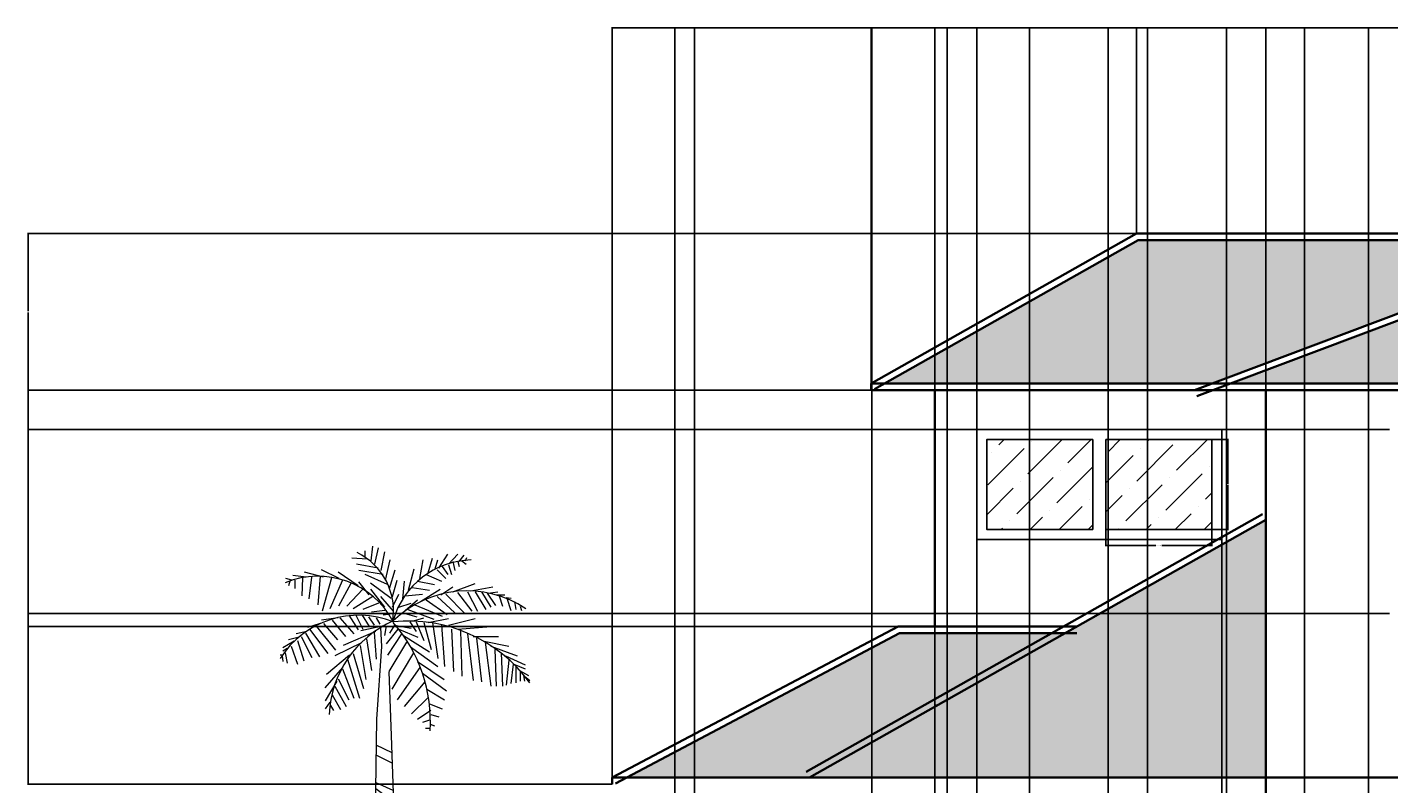
# Model space of a CAD drawing. Units: inches. Extents: x -177 to 697, y -125 to 346.
# Tile 2 of 4: x -177 to 237, y 116 to 346. Entities that reach past the tile are written whole.
import ezdxf

# ---------------------------------------------------------------- set-up
doc = ezdxf.new("R2010")
doc.units = ezdxf.units.IN
doc.header["$MEASUREMENT"] = 0
for name, color, linetype, lineweight in [('A-ANNO-DIMS', 2, 'Continuous', 18), ('A-GLAZ', 4, 'Continuous', 25), ('A-GLAZ-PATT', 252, 'Continuous', 13), ('A-ROOF', 1, 'Continuous', 35), ('A-ROOF-PATT', 252, 'Continuous', 13), ('A-WALL', 7, 'Continuous', 35), ('L-PLNT', 94, 'Continuous', 13)]:
    doc.layers.add(name, color=color, linetype=linetype, lineweight=lineweight)
doc.styles.get("Standard").update_dxf_attribs({"font": 'arial.ttf'})
doc.dimstyles.get("Standard").update_dxf_attribs({"dimtxt": 0.18, "dimasz": 0.18, "dimexe": 0.18, "dimexo": 0.0625, "dimgap": 0.09, "dimtad": 0, "dimtih": 1, "dimtoh": 1, "dimdec": 4, "dimzin": 0, "dimdsep": 46, "dimtxsty": 'Standard', "dimcen": 0.09, "dimadec": 0, "dimazin": 0, "dimtfac": 1, "dimtdec": 4, "dimtofl": 0, "dimtmove": 0, "dimatfit": 3, "dimfxl": 1, "dimtolj": 1, "dimtzin": 0, "dimarcsym": 0})

# ---------------------------------------------------------------- blocks, each defined once
blk = doc.blocks.new('*U2')
for p, q in [((-7.5, 199.68), (-7.5, 197.946)), ((-5.567, 196.707), (-4.987, 201.167)), ((-4.407, 195.716), (-3.247, 200.672)), ((-2.474, 193.733), (-1.315, 199.433)), ((-6.727, 197.202), (-11.366, 197.45)), ((-3.441, 194.477), (-10.013, 195.716)), ((-1.121, 190.759), (0.232, 196.955)), ((9.317, 191.255), (10.283, 196.955)), ((11.829, 192.99), (13.182, 197.45)), ((13.956, 194.229), (14.729, 196.955)), ((15.116, 194.477), (17.822, 198.689)), ((16.082, 194.972), (17.822, 192.494)), ((18.015, 195.716), (20.914, 198.689)), ((18.015, 195.468), (18.981, 192.494)), ((19.368, 196.459), (19.948, 193.733)), ((20.914, 196.459), (21.301, 194.972)), ((21.301, 196.459), (22.847, 198.441)), ((22.074, 196.707), (23.427, 195.716)), ((23.234, 196.707), (23.62, 197.698)), ((-29.729, 190.759), (-31.469, 191.255)), ((-25.283, 191.751), (-29.342, 192.246)), ((-28.763, 190.759), (-28.763, 188.281)), ((-26.443, 191.503), (-26.636, 186.051)), ((-20.064, 191.751), (-25.863, 193.238)), ((-23.737, 191.751), (-24.51, 185.06)), ((-21.031, 191.998), (-21.804, 183.325)), ((-15.232, 191.255), (-20.644, 193.981)), ((-17.551, 191.503), (-20.451, 181.343)), ((-14.265, 190.759), (-18.131, 182.086)), ((-9.433, 189.025), (-15.618, 193.238)), ((-1.894, 192.494), (-9.24, 193.733)), ((-0.541, 189.52), (-7.307, 192.494)), ((0.038, 188.281), (1.778, 193.981)), ((1.005, 185.803), (2.358, 190.759)), ((5.837, 187.786), (7.577, 194.229)), ((11.25, 192.494), (15.889, 190.512)), ((14.536, 193.981), (17.242, 191.255)), ((-30.309, 190.512), (-30.695, 189.025)), ((-11.753, 189.768), (-15.425, 182.83)), ((-8.08, 188.034), (-12.912, 182.83)), ((-6.147, 186.299), (-9.24, 190.264)), ((-5.76, 190.016), (0.618, 185.308)), ((-5.76, 188.034), (-1.508, 182.582)), ((4.098, 185.06), (4.678, 190.512)), ((6.997, 188.529), (12.216, 187.786)), ((8.544, 190.512), (13.763, 189.52)), ((9.51, 184.317), (15.502, 188.034)), ((15.695, 186.299), (19.368, 188.777)), ((19.368, 187.29), (26.133, 189.768)), ((20.721, 187.042), (25.167, 181.343)), ((23.814, 187.29), (26.907, 181.343)), ((24.78, 187.538), (31.546, 188.777)), ((26.133, 187.29), (29.419, 181.838)), ((28.066, 187.29), (30.966, 182.582)), ((29.806, 186.795), (32.319, 183.078)), ((29.999, 186.795), (33.092, 187.29)), ((-4.987, 185.803), (-10.979, 182.086)), ((-3.247, 183.821), (-8.08, 181.838)), ((-2.668, 185.803), (1.198, 181.343)), ((1.005, 182.582), (2.938, 186.547)), ((2.938, 182.582), (6.61, 183.821)), ((4.871, 186.051), (10.09, 186.547)), ((4.871, 181.591), (8.544, 184.812)), ((7.77, 183.325), (16.082, 179.856)), ((11.25, 184.812), (17.628, 180.352)), ((14.536, 185.803), (19.948, 180.847)), ((17.242, 186.547), (23.041, 180.599)), ((32.512, 186.299), (35.218, 186.299)), ((33.479, 186.051), (34.445, 182.83)), ((35.605, 185.556), (37.151, 185.308)), ((35.798, 185.308), (36.958, 181.591)), ((38.118, 184.317), (38.504, 181.838)), ((39.857, 182.83), (40.244, 181.591)), ((-15.618, 179.36), (-20.644, 178.617)), ((-17.358, 178.617), (-13.299, 173.661)), ((-15.038, 179.36), (-10.786, 174.404)), ((-12.332, 180.104), (-9.433, 175.643)), ((-10.206, 180.104), (-8.08, 175.891)), ((-8.273, 180.104), (-6.147, 176.635)), ((-6.34, 179.608), (-4.6, 177.13)), ((-1.315, 181.591), (-5.374, 181.095)), ((-4.021, 179.36), (-2.861, 177.378)), ((-0.348, 180.352), (-1.894, 180.104)), ((4.098, 180.847), (8.35, 179.608)), ((5.644, 181.838), (13.569, 178.865)), ((7.384, 178.369), (10.476, 179.36)), ((11.829, 177.874), (18.015, 179.113)), ((18.015, 177.13), (26.133, 179.113)), ((-25.09, 175.148), (-28.376, 174.404)), ((-25.476, 174.652), (-21.224, 167.466)), ((-21.031, 177.626), (-24.897, 176.387)), ((-24.317, 175.891), (-18.711, 168.457)), ((-22.191, 176.635), (-16.391, 169.448)), ((-20.064, 177.626), (-15.812, 172.67)), ((-4.214, 175.148), (-14.072, 170.935)), ((-1.701, 176.882), (-8.66, 175.396)), ((-4.6, 174.9), (-4.021, 166.722)), ((-2.668, 176.387), (-2.376, 170.594)), ((-0.928, 176.882), (-1.508, 173.909)), ((2.551, 175.891), (-0.928, 171.431)), ((3.711, 174.404), (-0.541, 167.961)), ((1.585, 177.13), (0.038, 174.652)), ((1.585, 177.13), (6.61, 176.139)), ((2.938, 175.891), (8.737, 173.413)), ((6.224, 178.121), (8.157, 175.148)), ((8.157, 178.121), (10.476, 172.422)), ((10.476, 177.874), (12.796, 169.696)), ((13.182, 177.874), (14.729, 166.97)), ((15.889, 177.13), (16.855, 164.492)), ((18.981, 175.891), (19.561, 163.005)), ((20.914, 175.891), (30.966, 176.635)), ((21.688, 175.396), (22.074, 161.518)), ((23.814, 174.404), (25.554, 160.279)), ((-28.956, 172.174), (-32.435, 170.192)), ((-27.409, 173.413), (-30.695, 172.67)), ((-29.922, 170.687), (-27.989, 165.235)), ((-27.989, 172.422), (-26.056, 166.227)), ((-26.829, 173.661), (-23.544, 167.218)), ((-8.466, 171.678), (-16.585, 167.713)), ((-8.853, 170.935), (-7.113, 160.527)), ((-6.92, 172.917), (-5.374, 163.253)), ((5.257, 171.926), (-0.155, 163.005)), ((4.291, 173.909), (12.216, 168.953)), ((6.417, 170.439), (14.729, 164.492)), ((25.554, 173.661), (33.285, 173.661)), ((26.52, 173.165), (28.066, 159.784)), ((28.839, 172.174), (36.378, 170.687)), ((29.226, 171.926), (30.966, 158.545)), ((30.966, 170.687), (38.891, 167.713)), ((-32.628, 167.961), (-33.208, 167.961)), ((-32.628, 167.713), (-32.435, 165.979)), ((-31.082, 169.944), (-32.435, 169.2)), ((-31.662, 168.705), (-31.082, 165.483)), ((-12.139, 167.961), (-19.098, 162.014)), ((-12.719, 166.722), (-9.046, 154.828)), ((-10.979, 168.457), (-7.887, 157.801)), ((7.384, 168.705), (0.812, 157.553)), ((8.544, 165.979), (16.662, 160.527)), ((32.126, 169.696), (32.512, 158.545)), ((34.058, 168.705), (34.445, 158.545)), ((35.412, 167.713), (41.404, 164.988)), ((36.378, 166.474), (35.605, 158.792)), ((-14.265, 164.244), (-19.678, 158.049)), ((-14.265, 163.749), (-10.786, 154.828)), ((9.317, 164.244), (2.358, 154.332)), ((10.09, 162.51), (17.435, 157.058)), ((37.731, 165.235), (36.958, 159.288)), ((37.924, 165.235), (41.404, 163.749)), ((38.504, 164.492), (38.504, 159.536)), ((39.664, 163.253), (42.37, 161.766)), ((39.857, 162.757), (39.857, 160.031)), ((40.824, 161.766), (41.21, 160.031)), ((-16.005, 160.031), (-19.484, 154.084)), ((-16.585, 158.545), (-13.106, 152.35)), ((-15.618, 160.775), (-12.332, 154.332)), ((10.863, 159.784), (4.484, 152.35)), ((11.443, 157.553), (16.855, 154.332)), ((41.21, 161.518), (42.757, 160.279)), ((-18.131, 153.589), (-19.484, 151.606)), ((-17.358, 155.819), (-14.845, 151.358)), ((11.829, 155.075), (6.804, 150.119)), ((-17.938, 152.597), (-16.972, 151.111)), ((12.603, 151.111), (8.544, 148.385)), ((12.216, 153.093), (16.082, 151.606)), ((12.603, 149.872), (15.116, 149.128)), ((12.216, 148.137), (10.09, 147.393)), ((12.409, 145.659), (11.056, 145.659)), ((12.409, 146.898), (13.763, 146.402)), ((-4.081, 140.645), (0.753, 138.261)), ((-4.081, 137.547), (0.753, 135.163)), ((-4.081, 129.205), (1.124, 126.821)), ((-4.081, 127.298), (1.31, 123.246)), ((-4.081, 121.578), (1.31, 120.863)), ((-4.453, 112.283), (1.682, 105.133)), ((-4.267, 114.428), (1.682, 108.708)), ((-4.639, 102.273), (1.868, 100.604)), ((-4.453, 99.651), (2.24, 98.459)), ((-4.453, 91.071), (2.426, 89.641)), ((-4.825, 83.921), (2.612, 81.061)), ((-4.639, 81.299), (2.797, 78.916)), ((-4.639, 78.916), (2.797, 76.771))]:
    blk.add_line(p, q)
for points in [[(-2.363, 170.553), (-3.88, 148.505), (-4.988, 69.634), (-3.325, 24.869), (0, 0)], [(-0.116, 162.848), (0.554, 143.532), (2.217, 96.635), (3.88, 44.054), (7.76, 12.079), (11.64, 0)]]:
    blk.add_lwpolyline(points)
for centre, radius, start, end in [((-18.427, 181.448), 19.715, 350.285, 64.11229), ((25.595, 171.567), 25.395, 91.40319, 163.882), ((-21.738, 166.094), 25.899, 27.67115, 112.5305), ((23.687, 155.341), 32.188, 56.19272, 134.3213), ((-9.259, 151.732), 28.386, 68.38311, 147.5322), ((14.394, 148.393), 32.752, 113.7592, 177.4133), ((5.828, 132.718), 45.639, 35.98777, 95.82273), ((-32.8, 147.923), 45.309, 356.1943, 41.37848)]:
    blk.add_arc(centre, radius, start, end)
blk = doc.blocks.new('WIN-SASH-UPPER-ELEV')
blk.add_line((0, 27.46), (0, 0))
blk.add_lwpolyline([(0, 27.46), (32.26, 27.46), (32.26, 0), (0, 0)])
blk = doc.blocks.new('*D13')
at = {"layer": 'A-ANNO-DIMS', "color": 0, "lineweight": -2, "transparency": 16777216}
for p, q in [((151.36, 193.16), (151.36, 188.2)), ((183.62, 193.16), (183.62, 188.2)), ((151.54, 188.38), (166.58, 188.38)), ((183.44, 188.38), (168.39, 188.38))]:
    blk.add_line(p, q, dxfattribs=at)
at = {"layer": 'A-ANNO-DIMS', "color": 0, "transparency": 16777216}
for points in [[(151.54, 188.41), (151.54, 188.35), (151.36, 188.38)], [(183.44, 188.41), (183.44, 188.35), (183.62, 188.38)]]:
    blk.add_solid(points, dxfattribs=at)
at = {"layer": 'Defpoints', "color": 0, "transparency": 16777216}
for p in [(151.36, 193.22), (183.62, 193.22), (183.62, 188.38)]:
    blk.add_point(p, dxfattribs=at)
at = {"layer": 'A-ANNO-DIMS', "color": 0, "transparency": 16777216, "insert": (167.49, 188.38), "char_height": 0.18, "attachment_point": 5}
blk.add_mtext('\\A1;SASH 32 TYP.', dxfattribs=at)
blk = doc.blocks.new('*D14')
at = {"layer": 'A-ANNO-DIMS', "color": 0, "lineweight": -2, "transparency": 16777216}
for p, q in [((183.68, 220.68), (188.64, 220.68)), ((188.46, 220.5), (188.46, 207.13)), ((188.46, 193.4), (188.46, 206.77)), ((183.68, 193.22), (188.64, 193.22))]:
    blk.add_line(p, q, dxfattribs=at)
at = {"layer": 'A-ANNO-DIMS', "color": 0, "transparency": 16777216}
for points in [[(188.43, 220.5), (188.49, 220.5), (188.46, 220.68)], [(188.43, 193.4), (188.49, 193.4), (188.46, 193.22)]]:
    blk.add_solid(points, dxfattribs=at)
at = {"layer": 'Defpoints', "color": 0, "transparency": 16777216}
for p in [(183.62, 220.68), (188.46, 220.68), (183.62, 193.22)]:
    blk.add_point(p, dxfattribs=at)
at = {"layer": 'A-ANNO-DIMS', "color": 0, "transparency": 16777216, "insert": (188.46, 206.95), "char_height": 0.18, "attachment_point": 5}
blk.add_mtext('\\A1;27 TYP.', dxfattribs=at)
blk = doc.blocks.new('*D21')
at = {"layer": 'A-ANNO-DIMS', "color": 0, "lineweight": -2, "transparency": 16777216}
for p, q in [((1.05, 117.74), (1.05, 346.22)), ((1.23, 346.04), (259.84, 346.04)), ((519.23, 346.04), (260.62, 346.04)), ((519.41, 117.74), (519.41, 346.22))]:
    blk.add_line(p, q, dxfattribs=at)
at = {"layer": 'A-ANNO-DIMS', "color": 0, "transparency": 16777216}
for points in [[(1.23, 346.07), (1.23, 346.01), (1.05, 346.04)], [(519.23, 346.07), (519.23, 346.01), (519.41, 346.04)]]:
    blk.add_solid(points, dxfattribs=at)
at = {"layer": 'Defpoints', "color": 0, "transparency": 16777216}
for p in [(519.41, 346.04), (1.05, 117.68), (519.41, 117.68)]:
    blk.add_point(p, dxfattribs=at)
at = {"layer": 'A-ANNO-DIMS', "color": 0, "transparency": 16777216, "insert": (260.23, 346.04), "char_height": 0.18, "attachment_point": 5}
blk.add_mtext('\\A1;518.4', dxfattribs=at)
blk = doc.blocks.new('*D22')
at = {"layer": 'A-ANNO-DIMS', "color": 0, "lineweight": -2, "transparency": 16777216}
for p, q in [((79.79, 235.68), (-176.98, 235.68)), ((-176.8, 235.5), (-176.8, 175.86)), ((-176.8, 115.86), (-176.8, 175.5)), ((0.99, 115.68), (-176.98, 115.68))]:
    blk.add_line(p, q, dxfattribs=at)
at = {"layer": 'A-ANNO-DIMS', "color": 0, "transparency": 16777216}
for points in [[(-176.83, 235.5), (-176.77, 235.5), (-176.8, 235.68)], [(-176.83, 115.86), (-176.77, 115.86), (-176.8, 115.68)]]:
    blk.add_solid(points, dxfattribs=at)
at = {"layer": 'Defpoints', "color": 0, "transparency": 16777216}
for p in [(79.85, 235.68), (-176.8, 115.68), (1.05, 115.68)]:
    blk.add_point(p, dxfattribs=at)
at = {"layer": 'A-ANNO-DIMS', "color": 0, "transparency": 16777216, "insert": (-176.8, 175.68), "char_height": 0.18, "attachment_point": 5}
blk.add_mtext('\\A1;120', dxfattribs=at)
blk = doc.blocks.new('*D24')
at = {"layer": 'A-ANNO-DIMS', "color": 0, "lineweight": -2, "transparency": 16777216}
for p, q in [((128.05, -16.26), (128.05, 346.22)), ((128.23, 346.04), (157.83, 346.04)), ((187.87, 346.04), (158.27, 346.04)), ((188.05, 19.74), (188.05, 346.22))]:
    blk.add_line(p, q, dxfattribs=at)
at = {"layer": 'A-ANNO-DIMS', "color": 0, "transparency": 16777216}
for points in [[(128.23, 346.07), (128.23, 346.01), (128.05, 346.04)], [(187.87, 346.07), (187.87, 346.01), (188.05, 346.04)]]:
    blk.add_solid(points, dxfattribs=at)
at = {"layer": 'Defpoints', "color": 0, "transparency": 16777216}
for p in [(188.05, 346.04), (188.05, 19.68), (128.05, -16.32)]:
    blk.add_point(p, dxfattribs=at)
at = {"layer": 'A-ANNO-DIMS', "color": 0, "transparency": 16777216, "insert": (158.05, 346.04), "char_height": 0.18, "attachment_point": 5}
blk.add_mtext('\\A1;60', dxfattribs=at)
blk = doc.blocks.new('*D25')
at = {"layer": 'A-ANNO-DIMS', "color": 0, "lineweight": -2, "transparency": 16777216}
for p, q in [((152.05, 1.74), (152.05, 346.22)), ((152.23, 346.04), (157.84, 346.04)), ((163.87, 346.04), (158.26, 346.04)), ((164.05, 1.74), (164.05, 346.22))]:
    blk.add_line(p, q, dxfattribs=at)
at = {"layer": 'A-ANNO-DIMS', "color": 0, "transparency": 16777216}
for points in [[(152.23, 346.07), (152.23, 346.01), (152.05, 346.04)], [(163.87, 346.07), (163.87, 346.01), (164.05, 346.04)]]:
    blk.add_solid(points, dxfattribs=at)
at = {"layer": 'Defpoints', "color": 0, "transparency": 16777216}
for p in [(164.05, 346.04), (152.05, 1.68), (164.05, 1.68)]:
    blk.add_point(p, dxfattribs=at)
at = {"layer": 'A-ANNO-DIMS', "color": 0, "transparency": 16777216, "insert": (158.05, 346.04), "char_height": 0.18, "attachment_point": 5}
blk.add_mtext('\\A1;12', dxfattribs=at)
blk = doc.blocks.new('*D28')
at = {"layer": 'A-ANNO-DIMS', "color": 0, "lineweight": -2, "transparency": 16777216}
for p, q in [((211.79, 58.26), (211.79, 346.22)), ((211.97, 346.04), (221.1, 346.04)), ((231.15, 346.04), (222.01, 346.04)), ((231.33, 58.26), (231.33, 346.22))]:
    blk.add_line(p, q, dxfattribs=at)
at = {"layer": 'A-ANNO-DIMS', "color": 0, "transparency": 16777216}
for points in [[(211.97, 346.07), (211.97, 346.01), (211.79, 346.04)], [(231.15, 346.07), (231.15, 346.01), (231.33, 346.04)]]:
    blk.add_solid(points, dxfattribs=at)
at = {"layer": 'Defpoints', "color": 0, "transparency": 16777216}
for p in [(231.33, 346.04), (211.79, 58.19), (231.33, 58.19)]:
    blk.add_point(p, dxfattribs=at)
at = {"layer": 'A-ANNO-DIMS', "color": 0, "transparency": 16777216, "insert": (221.56, 346.04), "char_height": 0.18, "attachment_point": 5}
blk.add_mtext('\\A1;19.536', dxfattribs=at)
blk = doc.blocks.new('*D29')
at = {"layer": 'A-ANNO-DIMS', "color": 0, "lineweight": -2, "transparency": 16777216}
for p, q in [((200.05, 235.74), (200.05, 346.22)), ((200.23, 346.04), (289.77, 346.04)), ((379.87, 346.04), (290.33, 346.04)), ((380.05, 235.74), (380.05, 346.22))]:
    blk.add_line(p, q, dxfattribs=at)
at = {"layer": 'A-ANNO-DIMS', "color": 0, "transparency": 16777216}
for points in [[(200.23, 346.07), (200.23, 346.01), (200.05, 346.04)], [(379.87, 346.07), (379.87, 346.01), (380.05, 346.04)]]:
    blk.add_solid(points, dxfattribs=at)
at = {"layer": 'Defpoints', "color": 0, "transparency": 16777216}
for p in [(380.05, 346.04), (200.05, 235.68), (380.05, 235.68)]:
    blk.add_point(p, dxfattribs=at)
at = {"layer": 'A-ANNO-DIMS', "color": 0, "transparency": 16777216, "insert": (290.05, 346.04), "char_height": 0.18, "attachment_point": 5}
blk.add_mtext('\\A1;180', dxfattribs=at)
blk = doc.blocks.new('*D31')
at = {"layer": 'A-ANNO-DIMS', "color": 0, "lineweight": -2, "transparency": 16777216}
for p, q in [((80.05, -16.26), (80.05, 346.22)), ((80.23, 346.04), (103.83, 346.04)), ((127.87, 346.04), (104.27, 346.04)), ((128.05, -16.26), (128.05, 346.22))]:
    blk.add_line(p, q, dxfattribs=at)
at = {"layer": 'A-ANNO-DIMS', "color": 0, "transparency": 16777216}
for points in [[(80.23, 346.07), (80.23, 346.01), (80.05, 346.04)], [(127.87, 346.07), (127.87, 346.01), (128.05, 346.04)]]:
    blk.add_solid(points, dxfattribs=at)
at = {"layer": 'Defpoints', "color": 0, "transparency": 16777216}
for p in [(128.05, 346.04), (80.05, -16.32), (128.05, -16.32)]:
    blk.add_point(p, dxfattribs=at)
at = {"layer": 'A-ANNO-DIMS', "color": 0, "transparency": 16777216, "insert": (104.05, 346.04), "char_height": 0.18, "attachment_point": 5}
blk.add_mtext('\\A1;48', dxfattribs=at)
blk = doc.blocks.new('*D34')
at = {"layer": 'A-ANNO-DIMS', "color": 0, "lineweight": -2, "transparency": 16777216}
for p, q in [((237.69, 223.68), (-176.98, 223.68)), ((-176.8, 223.5), (-176.8, 195.86)), ((-176.8, 167.85), (-176.8, 195.49)), ((237.69, 167.67), (-176.98, 167.67))]:
    blk.add_line(p, q, dxfattribs=at)
at = {"layer": 'A-ANNO-DIMS', "color": 0, "transparency": 16777216}
for points in [[(-176.83, 223.5), (-176.77, 223.5), (-176.8, 223.68)], [(-176.83, 167.85), (-176.77, 167.85), (-176.8, 167.67)]]:
    blk.add_solid(points, dxfattribs=at)
at = {"layer": 'Defpoints', "color": 0, "transparency": 16777216}
for p in [(-176.8, 223.68), (237.75, 223.68), (237.75, 167.67)]:
    blk.add_point(p, dxfattribs=at)
at = {"layer": 'A-ANNO-DIMS', "color": 0, "transparency": 16777216, "insert": (-176.8, 195.68), "char_height": 0.18, "attachment_point": 5}
blk.add_mtext('\\A1;56.01', dxfattribs=at)
blk = doc.blocks.new('*D38')
at = {"layer": 'A-ANNO-DIMS', "color": 0, "lineweight": -2, "transparency": 16777216}
for p, q in [((20.05, 19.74), (20.05, 346.22)), ((20.23, 346.04), (22.75, 346.04)), ((25.88, 346.04), (23.36, 346.04)), ((26.06, 66.12), (26.06, 346.22))]:
    blk.add_line(p, q, dxfattribs=at)
at = {"layer": 'A-ANNO-DIMS', "color": 0, "transparency": 16777216}
for points in [[(20.23, 346.07), (20.23, 346.01), (20.05, 346.04)], [(25.88, 346.07), (25.88, 346.01), (26.06, 346.04)]]:
    blk.add_solid(points, dxfattribs=at)
at = {"layer": 'Defpoints', "color": 0, "transparency": 16777216}
for p in [(26.06, 346.04), (26.06, 66.06), (20.05, 19.68)]:
    blk.add_point(p, dxfattribs=at)
at = {"layer": 'A-ANNO-DIMS', "color": 0, "transparency": 16777216, "insert": (23.05, 346.04), "char_height": 0.18, "attachment_point": 5}
blk.add_mtext('\\A1;6.01', dxfattribs=at)
blk = doc.blocks.new('*D39')
at = {"layer": 'A-ANNO-DIMS', "color": 0, "lineweight": -2, "transparency": 16777216}
for p, q in [((80.05, -16.26), (80.05, 346.22)), ((80.23, 346.04), (91.11, 346.04)), ((102.79, 346.04), (91.9, 346.04)), ((102.97, 56.7), (102.97, 346.22))]:
    blk.add_line(p, q, dxfattribs=at)
at = {"layer": 'A-ANNO-DIMS', "color": 0, "transparency": 16777216}
for points in [[(80.23, 346.07), (80.23, 346.01), (80.05, 346.04)], [(102.79, 346.07), (102.79, 346.01), (102.97, 346.04)]]:
    blk.add_solid(points, dxfattribs=at)
at = {"layer": 'Defpoints', "color": 0, "transparency": 16777216}
for p in [(102.97, 346.04), (102.97, 56.63), (80.05, -16.32)]:
    blk.add_point(p, dxfattribs=at)
at = {"layer": 'A-ANNO-DIMS', "color": 0, "transparency": 16777216, "insert": (91.51, 346.04), "char_height": 0.18, "attachment_point": 5}
blk.add_mtext('\\A1;22.92', dxfattribs=at)
blk = doc.blocks.new('*D43')
at = {"layer": 'A-ANNO-DIMS', "color": 0, "lineweight": -2, "transparency": 16777216}
for p, q in [((99.22, 235.74), (99.22, 346.22)), ((99.4, 346.04), (105.2, 346.04)), ((111.92, 346.04), (106.11, 346.04)), ((112.1, 223.74), (112.1, 346.22))]:
    blk.add_line(p, q, dxfattribs=at)
at = {"layer": 'A-ANNO-DIMS', "color": 0, "transparency": 16777216}
for points in [[(99.4, 346.07), (99.4, 346.01), (99.22, 346.04)], [(111.92, 346.07), (111.92, 346.01), (112.1, 346.04)]]:
    blk.add_solid(points, dxfattribs=at)
at = {"layer": 'Defpoints', "color": 0, "transparency": 16777216}
for p in [(112.1, 346.04), (99.22, 235.68), (112.1, 223.68)]:
    blk.add_point(p, dxfattribs=at)
at = {"layer": 'A-ANNO-DIMS', "color": 0, "transparency": 16777216, "insert": (105.66, 346.04), "char_height": 0.18, "attachment_point": 5}
blk.add_mtext('\\A1;12.878', dxfattribs=at)
blk = doc.blocks.new('*D46')
at = {"layer": 'A-ANNO-DIMS', "color": 0, "lineweight": -2, "transparency": 16777216}
for p, q in [((112.1, 190.16), (112.1, -124.85)), ((186.62, 190.16), (186.62, -124.85)), ((112.28, -124.67), (148.96, -124.67)), ((186.44, -124.67), (149.75, -124.67))]:
    blk.add_line(p, q, dxfattribs=at)
at = {"layer": 'A-ANNO-DIMS', "color": 0, "transparency": 16777216}
for points in [[(112.28, -124.64), (112.28, -124.7), (112.1, -124.67)], [(186.44, -124.64), (186.44, -124.7), (186.62, -124.67)]]:
    blk.add_solid(points, dxfattribs=at)
at = {"layer": 'Defpoints', "color": 0, "transparency": 16777216}
for p in [(112.1, 190.22), (186.62, 190.22), (186.62, -124.67)]:
    blk.add_point(p, dxfattribs=at)
at = {"layer": 'A-ANNO-DIMS', "color": 0, "transparency": 16777216, "insert": (149.36, -124.67), "char_height": 0.18, "attachment_point": 5}
blk.add_mtext('\\A1;74.52', dxfattribs=at)
blk = doc.blocks.new('*D47')
at = {"layer": 'A-ANNO-DIMS', "color": 0, "lineweight": -2, "transparency": 16777216}
for p, q in [((160.63, 283.45), (160.63, 346.22)), ((160.81, 346.04), (224.99, 346.04)), ((290.08, 346.04), (225.9, 346.04)), ((290.26, 283.45), (290.26, 346.22))]:
    blk.add_line(p, q, dxfattribs=at)
at = {"layer": 'A-ANNO-DIMS', "color": 0, "transparency": 16777216}
for points in [[(160.81, 346.07), (160.81, 346.01), (160.63, 346.04)], [(290.08, 346.07), (290.08, 346.01), (290.26, 346.04)]]:
    blk.add_solid(points, dxfattribs=at)
at = {"layer": 'Defpoints', "color": 0, "transparency": 16777216}
for p in [(290.26, 346.04), (160.63, 283.39), (290.26, 283.39)]:
    blk.add_point(p, dxfattribs=at)
at = {"layer": 'A-ANNO-DIMS', "color": 0, "transparency": 16777216, "insert": (225.44, 346.04), "char_height": 0.18, "attachment_point": 5}
blk.add_mtext('\\A1;129.63', dxfattribs=at)
blk = doc.blocks.new('*D49')
at = {"layer": 'A-ANNO-DIMS', "color": 0, "lineweight": -2, "transparency": 16777216}
for p, q in [((160.57, 283.39), (-176.98, 283.39)), ((-176.8, 283.21), (-176.8, 259.72)), ((-176.8, 235.86), (-176.8, 259.35)), ((79.79, 235.68), (-176.98, 235.68))]:
    blk.add_line(p, q, dxfattribs=at)
at = {"layer": 'A-ANNO-DIMS', "color": 0, "transparency": 16777216}
for points in [[(-176.83, 283.21), (-176.77, 283.21), (-176.8, 283.39)], [(-176.83, 235.86), (-176.77, 235.86), (-176.8, 235.68)]]:
    blk.add_solid(points, dxfattribs=at)
at = {"layer": 'Defpoints', "color": 0, "transparency": 16777216}
for p in [(-176.8, 283.39), (160.63, 283.39), (79.85, 235.68)]:
    blk.add_point(p, dxfattribs=at)
at = {"layer": 'A-ANNO-DIMS', "color": 0, "transparency": 16777216, "insert": (-176.8, 259.53), "char_height": 0.18, "attachment_point": 5}
blk.add_mtext('\\A1;47.71', dxfattribs=at)
blk = doc.blocks.new('*D51')
at = {"layer": 'A-ANNO-DIMS', "color": 0, "lineweight": -2, "transparency": 16777216}
for p, q in [((99.22, 235.62), (99.22, -124.85)), ((200.05, 235.62), (200.05, -124.85)), ((99.4, -124.67), (149.18, -124.67)), ((199.87, -124.67), (150.09, -124.67))]:
    blk.add_line(p, q, dxfattribs=at)
at = {"layer": 'A-ANNO-DIMS', "color": 0, "transparency": 16777216}
for points in [[(99.4, -124.64), (99.4, -124.7), (99.22, -124.67)], [(199.87, -124.64), (199.87, -124.7), (200.05, -124.67)]]:
    blk.add_solid(points, dxfattribs=at)
at = {"layer": 'Defpoints', "color": 0, "transparency": 16777216}
for p in [(99.22, 235.68), (200.05, 235.68), (200.05, -124.67)]:
    blk.add_point(p, dxfattribs=at)
at = {"layer": 'A-ANNO-DIMS', "color": 0, "transparency": 16777216, "insert": (149.63, -124.67), "char_height": 0.18, "attachment_point": 5}
blk.add_mtext('\\A1;100.83', dxfattribs=at)
blk = doc.blocks.new('*D52')
at = {"layer": 'A-ANNO-DIMS', "color": 0, "lineweight": -2, "transparency": 16777216}
for p, q in [((79.85, 237.74), (79.85, 346.22)), ((80.03, 346.04), (119.85, 346.04)), ((160.45, 346.04), (120.64, 346.04)), ((160.63, 283.45), (160.63, 346.22))]:
    blk.add_line(p, q, dxfattribs=at)
at = {"layer": 'A-ANNO-DIMS', "color": 0, "transparency": 16777216}
for points in [[(80.03, 346.07), (80.03, 346.01), (79.85, 346.04)], [(160.45, 346.07), (160.45, 346.01), (160.63, 346.04)]]:
    blk.add_solid(points, dxfattribs=at)
at = {"layer": 'Defpoints', "color": 0, "transparency": 16777216}
for p in [(160.63, 346.04), (160.63, 283.39), (79.85, 237.68)]:
    blk.add_point(p, dxfattribs=at)
at = {"layer": 'A-ANNO-DIMS', "color": 0, "transparency": 16777216, "insert": (120.24, 346.04), "char_height": 0.18, "attachment_point": 5}
blk.add_mtext('\\A1;80.77', dxfattribs=at)
blk = doc.blocks.new('*D54')
at = {"layer": 'A-ANNO-DIMS', "color": 0, "lineweight": -2, "transparency": 16777216}
for p, q in [((99.16, 235.68), (-176.98, 235.68)), ((-176.8, 235.5), (-176.8, 199.86)), ((-176.8, 163.86), (-176.8, 199.5)), ((99.16, 163.68), (-176.98, 163.68))]:
    blk.add_line(p, q, dxfattribs=at)
at = {"layer": 'A-ANNO-DIMS', "color": 0, "transparency": 16777216}
for points in [[(-176.83, 235.5), (-176.77, 235.5), (-176.8, 235.68)], [(-176.83, 163.86), (-176.77, 163.86), (-176.8, 163.68)]]:
    blk.add_solid(points, dxfattribs=at)
at = {"layer": 'Defpoints', "color": 0, "transparency": 16777216}
for p in [(-176.8, 235.68), (99.22, 235.68), (99.22, 163.68)]:
    blk.add_point(p, dxfattribs=at)
at = {"layer": 'A-ANNO-DIMS', "color": 0, "transparency": 16777216, "insert": (-176.8, 199.68), "char_height": 0.18, "attachment_point": 5}
blk.add_mtext('\\A1;72', dxfattribs=at)
blk = doc.blocks.new('*D55')
at = {"layer": 'A-ANNO-DIMS', "color": 0, "lineweight": -2, "transparency": 16777216}
for p, q in [((20.05, 115.74), (20.05, 346.22)), ((20.23, 346.04), (59.24, 346.04)), ((99.04, 346.04), (60.03, 346.04)), ((99.22, 163.74), (99.22, 346.22))]:
    blk.add_line(p, q, dxfattribs=at)
at = {"layer": 'A-ANNO-DIMS', "color": 0, "transparency": 16777216}
for points in [[(20.23, 346.07), (20.23, 346.01), (20.05, 346.04)], [(99.04, 346.07), (99.04, 346.01), (99.22, 346.04)]]:
    blk.add_solid(points, dxfattribs=at)
at = {"layer": 'Defpoints', "color": 0, "transparency": 16777216}
for p in [(99.22, 346.04), (99.22, 163.68), (20.05, 115.68)]:
    blk.add_point(p, dxfattribs=at)
at = {"layer": 'A-ANNO-DIMS', "color": 0, "transparency": 16777216, "insert": (59.63, 346.04), "char_height": 0.18, "attachment_point": 5}
blk.add_mtext('\\A1;79.17', dxfattribs=at)

msp = doc.modelspace()

# ---------------------------------------------------------------- hatches: boundary and pattern name
at = {"layer": 'A-GLAZ-PATT'}
h = msp.add_hatch(dxfattribs=at)
h.set_pattern_fill('ANSI36', color=256, scale=50)
h.set_pattern_definition([(45, (-118.808, -115.7344), (3.31456, 12.1534), [15.625, -3.125, 0, -3.125])])
h.paths.add_polyline_path([(183.617, 220.6802), (151.3569, 220.6802), (151.3569, 193.2226), (183.617, 193.2226)])
h.paths.add_polyline_path([(147.3569, 220.6802), (115.0968, 220.6802), (115.0968, 193.2226), (147.3569, 193.2226)])
at = {"layer": 'A-ROOF-PATT'}
h = msp.add_hatch(dxfattribs=at)
h.set_pattern_fill('AR-BRSTD', color=256)
h.set_pattern_definition([(0, (-118.8082, -115.7344), (0, 2.667), []), (90, (-118.808, -115.7344), (-4, 2.667), [2.667, -2.667])])
h.paths.add_polyline_path([(289.952, 277.6802), (396.2807, 237.6802), (500.0496, 237.6802), (514.1115, 237.6802), (351.0539, 304.0916), (290.6192, 281.3896), (161.1548, 281.3896), (83.9154, 237.6802), (183.6234, 237.6802)])
h.paths.add_polyline_path([(289.952, 275.5434), (189.3036, 237.6802), (390.6005, 237.6802)], flags=17)
h.paths.add_polyline_path([(200.0496, 196.199), (61.0496, 117.6802), (200.0496, 117.6802)])
h.paths.add_polyline_path([(88.5518, 161.6802), (5.3286, 117.6802), (61.0496, 117.6802), (138.9418, 161.6802)])
h.paths.add_polyline_path([(380.0496, 191.2819), (380.0496, 117.6802), (500.0496, 117.6802), (500.0496, 125.9461)])

# ---------------------------------------------------------------- linework, layer by layer
at = {"layer": 'A-GLAZ'}
msp.add_lwpolyline([(112.0968, 223.6802), (186.617, 223.6802), (186.617, 190.2226), (112.0968, 190.2226)], close=True, dxfattribs=at)
at = {"layer": 'A-ROOF'}
for p, q in [((79.8545, 237.6802), (500.0496, 237.6802)), ((79.8545, 237.6802), (79.8545, 235.6802)), ((79.8545, 235.6802), (500.0496, 235.6802)), ((60.0659, 119.4216), (199.0659, 197.9404)), ((61.0496, 117.6802), (200.0496, 196.199)), ((200.0496, 196.199), (200.0496, 196.199)), ((99.2186, 139.6802), (99.9957, 139.6802)), ((1.0496, 117.6802), (500.0496, 117.6802)), ((1.0496, 117.6802), (1.0496, 115.6802))]:
    msp.add_line(p, q, dxfattribs=at)
for points in [[(79.8545, 237.6802), (160.6282, 283.3896), (290.2559, 283.3896), (351.0833, 306.2391), (519.4137, 237.6802)], [(80.8395, 235.9396), (161.1548, 281.3896), (290.6192, 281.3896), (351.0539, 304.0916), (518.6593, 235.828)], [(178.307, 235.6802), (289.952, 277.6802), (401.5971, 235.6802)], [(179.0112, 233.8083), (289.952, 275.5434), (400.8929, 233.8083)], [(142.4823, 163.6802), (88.0556, 163.6802), (88.0556, 163.6802), (1.0496, 117.6802)], [(142.4823, 161.6802), (88.5518, 161.6802), (1.9844, 115.9122)]]:
    msp.add_lwpolyline(points, dxfattribs=at)
at = {"layer": 'A-WALL'}
for p, q in [((99.2186, 163.6802), (99.2186, 235.6802)), ((200.0496, -16.3198), (200.0496, 235.6802))]:
    msp.add_line(p, q, dxfattribs=at)

# ---------------------------------------------------------------- block references
at = {"layer": 'A-GLAZ', "rotation": 180}
msp.add_blockref('WIN-SASH-UPPER-ELEV', (147.3569, 220.6802), dxfattribs=at)
at = {"layer": 'A-GLAZ'}
msp.add_blockref('WIN-SASH-UPPER-ELEV', (151.3569, 193.2226), dxfattribs=at)
at = {"layer": 'L-PLNT'}
msp.add_blockref('*U2', (-66.8579, -12.984), dxfattribs=at)

# ---------------------------------------------------------------- dimensions: what is measured, and where the dimension line sits
at = {"layer": 'A-ANNO-DIMS'}
for base, p1, p2, override, picture, middle in [((519.4137, 346.0391), (1.0496, 117.6802), (519.4137, 117.6802), {"dimdec": 1, "dimlfac": 1, "dimrnd": 0, "dimzin": 0, "dimdsep": 46, "dimlunit": 2}, '*D21', (260.2316, 346.0391)), ((26.0592, 346.0391), (20.0496, 19.6802), (26.0592, 66.059), {"dimdec": 2, "dimlfac": 1, "dimrnd": 0, "dimzin": 0, "dimdsep": 46, "dimlunit": 2}, '*D38', (23.0544, 346.0391)), ((99.2186, 346.0391), (20.0496, 115.6802), (99.2186, 163.6802), {"dimdec": 2, "dimlfac": 1, "dimrnd": 0, "dimzin": 0, "dimdsep": 46, "dimlunit": 2}, '*D55', (59.6341, 346.0391)), ((160.6282, 346.0391), (79.8545, 237.6802), (160.6282, 283.3896), {"dimdec": 2, "dimlfac": 1, "dimrnd": 0, "dimzin": 0, "dimdsep": 46, "dimlunit": 2}, '*D52', (120.2413, 346.0391)), ((128.0496, 346.0391), (80.0496, -16.3198), (128.0496, -16.3198), {"dimdec": 0, "dimlfac": 1, "dimrnd": 0, "dimzin": 0, "dimdsep": 46, "dimlunit": 2}, '*D31', (104.0496, 346.0391)), ((102.9675, 346.0391), (80.0496, -16.3198), (102.9675, 56.6343), {"dimdec": 2, "dimlfac": 1, "dimrnd": 0, "dimzin": 0, "dimdsep": 46, "dimlunit": 2}, '*D39', (91.5085, 346.0391)), ((112.0968, 346.0391), (99.2186, 235.6802), (112.0968, 223.6802), {"dimdec": 3, "dimlfac": 1, "dimrnd": 0, "dimzin": 0, "dimdsep": 46, "dimlunit": 2}, '*D43', (105.6577, 346.0391)), ((188.0496, 346.0391), (128.0496, -16.3198), (188.0496, 19.6802), {"dimdec": 0, "dimlfac": 1, "dimrnd": 0, "dimzin": 0, "dimdsep": 46, "dimlunit": 2}, '*D24', (158.0496, 346.0391)), ((164.0496, 346.0391), (152.0496, 1.6802), (164.0496, 1.6802), {"dimdec": 0, "dimlfac": 1, "dimrnd": 0, "dimzin": 0, "dimdsep": 46, "dimlunit": 2}, '*D25', (158.0496, 346.0391)), ((290.2559, 346.0391), (160.6282, 283.3896), (290.2559, 283.3896), {"dimdec": 2, "dimlfac": 1, "dimrnd": 0, "dimzin": 0, "dimdsep": 46, "dimlunit": 2}, '*D47', (225.442, 346.0391)), ((380.0496, 346.0391), (200.0496, 235.6802), (380.0496, 235.6802), {"dimdec": 0, "dimlfac": 1, "dimrnd": 0, "dimzin": 0, "dimdsep": 46, "dimlunit": 2}, '*D29', (290.0496, 346.0391)), ((231.32629, 346.03909), (211.78981, 58.1928), (231.32629, 58.1928), {"dimdec": 3, "dimlfac": 1, "dimrnd": 0, "dimzin": 0, "dimdsep": 46, "dimlunit": 2}, '*D28', (221.55805, 346.03909)), ((200.0496, -124.671), (99.2186, 235.6802), (200.0496, 235.6802), {"dimdec": 2, "dimlfac": 1, "dimrnd": 0, "dimzin": 0, "dimdsep": 46, "dimlunit": 2}, '*D51', (149.6341, -124.671)), ((186.617, -124.671), (112.0968, 190.2226), (186.617, 190.2226), {"dimdec": 2, "dimlfac": 1, "dimrnd": 0, "dimzin": 0, "dimdsep": 46, "dimlunit": 2}, '*D46', (149.3569, -124.671))]:
    dim = msp.add_linear_dim(base=base, p1=p1, p2=p2, dimstyle='Standard', override=override, dxfattribs=at)
    dim.commit()
    dim.dimension.update_dxf_attribs({"geometry": picture, "text_midpoint": middle})
for base, p1, p2, override, picture, middle in [((-176.8039, 283.3896), (79.8545, 235.6802), (160.6282, 283.3896), {"dimdec": 2, "dimlfac": 1, "dimrnd": 0, "dimzin": 0, "dimdsep": 46, "dimlunit": 2}, '*D49', (-176.8039, 259.5349)), ((-176.8039, 115.6802), (79.8545, 235.6802), (1.0496, 115.6802), {"dimdec": 0, "dimlfac": 1, "dimrnd": 0, "dimzin": 0, "dimdsep": 46, "dimlunit": 2}, '*D22', (-176.8039, 175.6802)), ((-176.8039, 235.6802), (99.2186, 163.6802), (99.2186, 235.6802), {"dimdec": 0, "dimlfac": 1, "dimrnd": 0, "dimzin": 0, "dimdsep": 46, "dimlunit": 2}, '*D54', (-176.8039, 199.6802)), ((-176.8039, 223.6802), (237.7524, 167.6715), (237.7524, 223.6802), {"dimdec": 2, "dimlfac": 1, "dimrnd": 0, "dimzin": 0, "dimdsep": 46, "dimlunit": 2}, '*D34', (-176.8039, 195.6759))]:
    dim = msp.add_linear_dim(base=base, p1=p1, p2=p2, angle=90, dimstyle='Standard', override=override, dxfattribs=at)
    dim.commit()
    dim.dimension.update_dxf_attribs({"geometry": picture, "text_midpoint": middle})
dim = msp.add_linear_dim(base=(188.456, 220.6802), p1=(183.617, 193.2226), p2=(183.617, 220.6802), angle=90, text='<> TYP.', dimstyle='Standard', override={"dimdec": 0, "dimlfac": 1, "dimrnd": 0, "dimzin": 0, "dimdsep": 46, "dimlunit": 2}, dxfattribs=at)
dim.commit()
dim.dimension.update_dxf_attribs({"geometry": '*D14', "text_midpoint": (188.456, 206.9514)})
dim = msp.add_linear_dim(base=(183.617, 188.3836), p1=(151.3569, 193.2226), p2=(183.617, 193.2226), text='SASH <> TYP.', dimstyle='Standard', override={"dimdec": 0, "dimlfac": 1, "dimrnd": 0, "dimzin": 0, "dimdsep": 46, "dimlunit": 2}, dxfattribs=at)
dim.commit()
dim.dimension.update_dxf_attribs({"geometry": '*D13', "text_midpoint": (167.4869, 188.3836)})

doc.saveas('drawing.dxf')
